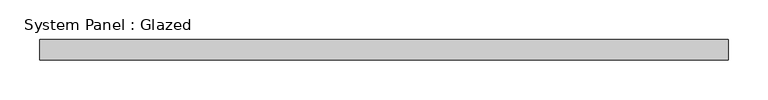
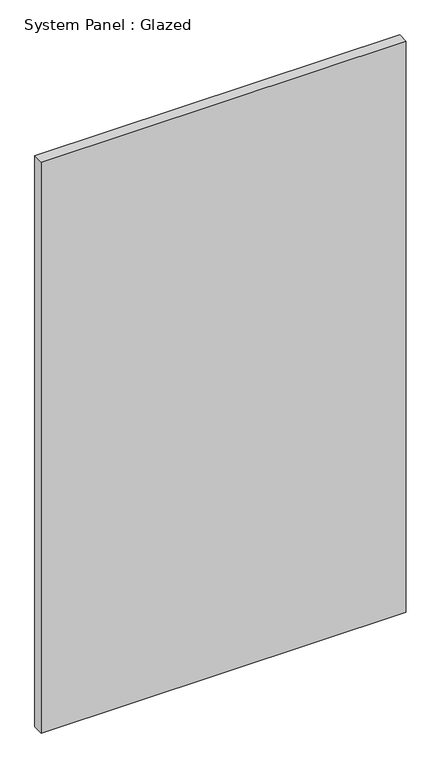
"""IFC4 building model written with IfcOpenShell, lengths in millimetres: plate geometry, System Panel : Glazed."""

from ifc_helpers import new_model, si_unit, origin, origin_with_axes, place, context, project, spatial, polyline, outline, extrude, source, transform, mapped, element, save


def system_panel_glazed_e33957fc(model_context):
    return source(origin(), model_context, "Body", "SweptSolid", [
        extrude(outline(polyline([(432.3220098, 19.05), (-432.3220098, 19.05), (-432.3220098, 44.45), (432.3220098, 44.45), (432.3220098, 19.05)])), origin_with_axes(), (0.0, 0.0, 1.0), 1428.75),
    ])


if __name__ == "__main__":
    model = new_model("IFC4")
    model_context = context("Model", 3, world=origin())
    ifc_project = project(units=[si_unit("LENGTHUNIT", "METRE", prefix="MILLI")], contexts=[model_context])
    site = spatial("IfcSite", under=ifc_project)
    building = spatial("IfcBuilding", under=site)
    placement = place(None, origin())
    system_panel_glazed_shape = system_panel_glazed_e33957fc(model_context)
    element("IfcPlate", 1, ObjectType="System Panel : Glazed", at=placement, inside=building, context=model_context, shape_type="MappedRepresentation", body=[
        mapped(system_panel_glazed_shape, transform((0.0, 0.0, 0.0), x_axis=(1.0, 0.0, 0.0), y_axis=(0.0, 1.0, 0.0), z_axis=(0.0, 0.0, 1.0))),
    ])
    save(model, "model.ifc")

# Revit data of these elements
# Type "System Panel : Glazed"
#   Construction Type Id = "GSP4R"
#   Analytic Construction = "1/8 in Pilkington single glazing"
#   Visual Light Transmittance = 0.9
#   Solar Heat Gain Coefficient = 0.86
#   Heat Transfer Coefficient (U) = 1.18115 BTU/(h·ft²·°F)
#   Define Thermal Properties by = 1
# Element 1 (IfcPlate, "System Panel : Glazed")
#   Materials on its faces: "Glass"
# Materials
#   "Glass": class "Glass", colour RGB 0 128 192, transparency 0.75, Description = "Soda Lime Glass", Cost = 0
